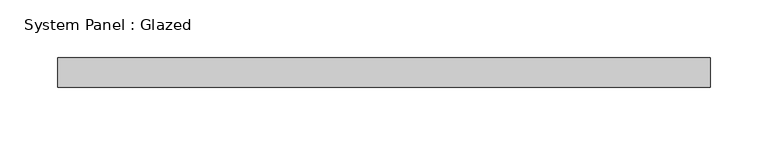
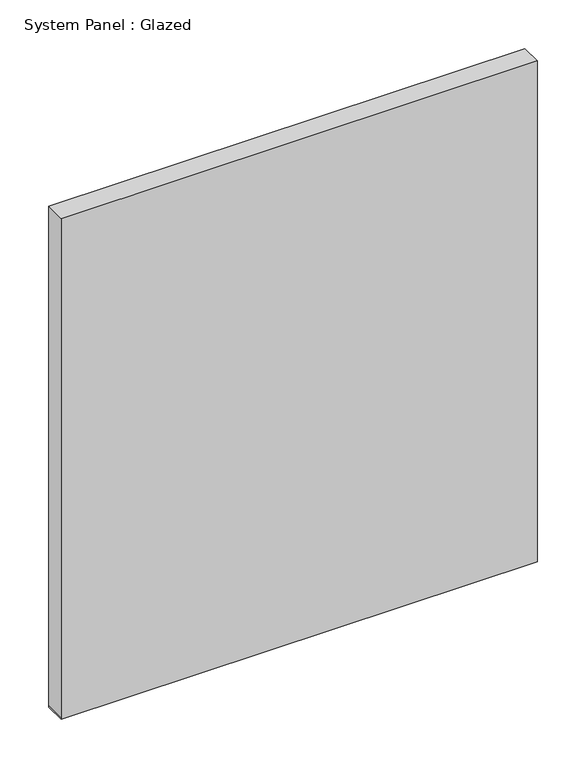
"""IFC4 building model written with IfcOpenShell, lengths in millimetres: plate geometry, System Panel : Glazed."""

from ifc_helpers import new_model, si_unit, frame, origin, place, context, project, spatial, polyline, outline, extrude, source, transform, mapped, element, save


def system_panel_glazed_31c741ab(model_context):
    return source(origin(), model_context, "Body", "SweptSolid", [
        extrude(outline(polyline([(0.0, -282.575), (0.0, 282.575), (2.1166667, 282.575), (628.3108298, 282.575), (628.3108298, -282.575), (2.1166667, -282.575), (0.0, -282.575)])), frame((0.0, 19.05, 0.0), z_axis=(0.0, 1.0, 0.0), x_axis=(0.0, 0.0, 1.0)), (0.0, 0.0, 1.0), 25.4),
    ])


if __name__ == "__main__":
    model = new_model("IFC4")
    model_context = context("Model", 3, world=origin())
    ifc_project = project(units=[si_unit("LENGTHUNIT", "METRE", prefix="MILLI")], contexts=[model_context])
    site = spatial("IfcSite", under=ifc_project)
    building = spatial("IfcBuilding", under=site)
    placement = place(None, origin())
    system_panel_glazed_shape = system_panel_glazed_31c741ab(model_context)
    element("IfcPlate", 1, ObjectType="System Panel : Glazed", at=placement, inside=building, context=model_context, shape_type="MappedRepresentation", body=[
        mapped(system_panel_glazed_shape, transform((0.0, 0.0, 0.0), x_axis=(1.0, 0.0, 0.0), y_axis=(0.0, 1.0, 0.0), z_axis=(0.0, 0.0, 1.0))),
    ])
    save(model, "model.ifc")

# Revit data of these elements
# Type "System Panel : Glazed"
#   Construction Type Id = "GSP4R"
#   Analytic Construction = "1/8 in Pilkington single glazing"
#   Visual Light Transmittance = 0.9
#   Solar Heat Gain Coefficient = 0.86
#   Heat Transfer Coefficient (U) = 1.18115 BTU/(h·ft²·°F)
#   Define Thermal Properties by = 1
# Element 1 (IfcPlate, "System Panel : Glazed")
#   Materials on its faces: "Glass"
# Materials
#   "Glass": class "Glass", colour RGB 0 128 192, transparency 0.75, Description = "Soda Lime Glass", Cost = 0
